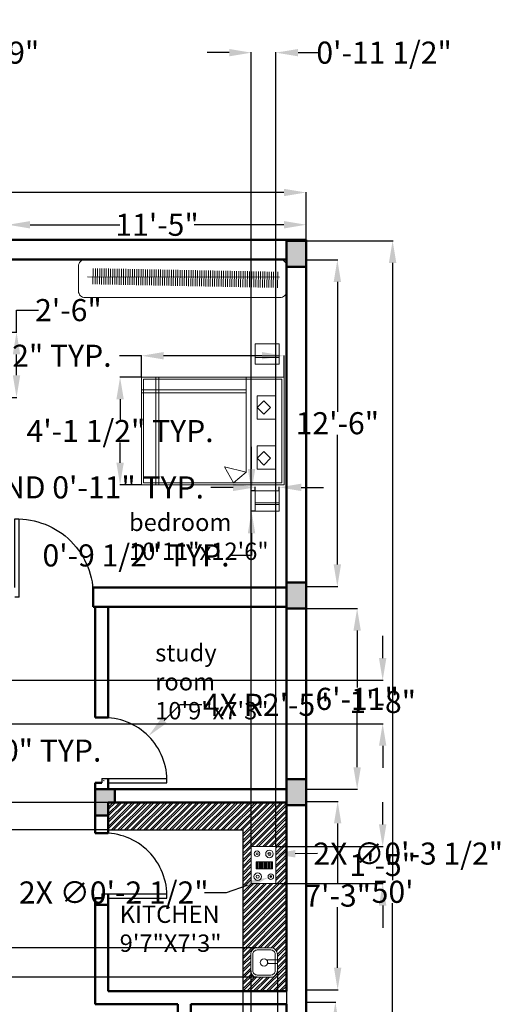
# Model space of a CAD drawing. Units: inches. Extents: x 22 to 1000, y 8 to 1043.
# Tile 3 of 3: x 779 to 1000, y 590 to 1043. Entities that reach past the tile are written whole.
import ezdxf

# ---------------------------------------------------------------- set-up
doc = ezdxf.new("R2010")
doc.units = ezdxf.units.IN
doc.header["$MEASUREMENT"] = 0
for name, color, linetype, lineweight in [('A-ANNO-DIMS', 2, 'Continuous', 18), ('A-AREA-IDEN', 7, 'Continuous', 25), ('A-COLS', 7, 'Continuous', 50), ('A-COLS-PATT', 1, 'Continuous', 13), ('A-CSWK', 30, 'Continuous', 25), ('A-DOOR', 4, 'Continuous', 25), ('A-EQPM', 9, 'Continuous', 18), ('A-EQPM-PATT', 9, 'Continuous', 13), ('A-FLOR-FIXT', 9, 'Continuous', 18), ('A-FURN', 8, 'Continuous', 18), ('A-FURN-PATT', 8, 'Continuous', 13), ('A-WALL', 7, 'Continuous', 50)]:
    doc.layers.add(name, color=color, linetype=linetype, lineweight=lineweight)
doc.layers.add('A-CSWK-PATT', color=143, linetype='Continuous', lineweight=13, true_color=0x7aafdf)
doc.styles.get("Standard").update_dxf_attribs({"font": 'arial.ttf'})
doc.dimstyles.get("Standard").update_dxf_attribs({"dimtxt": 10.18, "dimasz": 10.18, "dimexe": 0.18, "dimexo": 0.0625, "dimgap": 0.09, "dimtad": 0, "dimtih": 1, "dimtoh": 1, "dimdec": 0, "dimzin": 0, "dimdsep": 46, "dimlunit": 3, "dimtxsty": 'Standard', "dimcen": 0.09, "dimadec": 0, "dimazin": 0, "dimtfac": 1, "dimtdec": 0, "dimtofl": 0, "dimtmove": 0, "dimatfit": 3, "dimfxl": 1, "dimtolj": 1, "dimtzin": 0, "dimarcsym": 0})

# ---------------------------------------------------------------- blocks, each defined once
blk = doc.blocks.new('*D7')
at = {"layer": 'A-ANNO-DIMS', "color": 0, "lineweight": -2, "transparency": 16777216}
for p, q in [((773.8, 941.72), (773.8, 948.83)), ((783.98, 948.65), (825.3, 948.65)), ((900.81, 948.65), (859.49, 948.65)), ((910.99, 941.72), (910.99, 948.83))]:
    blk.add_line(p, q, dxfattribs=at)
at = {"layer": 'A-ANNO-DIMS', "color": 0, "transparency": 16777216}
for points in [[(783.98, 950.35), (783.98, 946.95), (773.8, 948.65)], [(900.81, 950.35), (900.81, 946.95), (910.99, 948.65)]]:
    blk.add_solid(points, dxfattribs=at)
at = {"layer": 'Defpoints', "color": 0, "transparency": 16777216}
for p in [(910.99, 948.65), (773.8, 941.66), (910.99, 941.66)]:
    blk.add_point(p, dxfattribs=at)
at = {"layer": 'A-ANNO-DIMS', "color": 0, "transparency": 16777216, "insert": (842.39, 948.65), "char_height": 10.18, "attachment_point": 5}
blk.add_mtext('\\A1;11\'-5"', dxfattribs=at)
blk = doc.blocks.new('*D14')
at = {"layer": 'A-ANNO-DIMS', "color": 0, "lineweight": -2, "transparency": 16777216}
for p, q in [((911.05, 590.68), (924.64, 590.68)), ((924.46, 580.5), (924.46, 471.45)), ((924.46, 351.84), (924.46, 460.88)), ((911.05, 341.66), (924.64, 341.66))]:
    blk.add_line(p, q, dxfattribs=at)
at = {"layer": 'A-ANNO-DIMS', "color": 0, "transparency": 16777216}
for points in [[(922.77, 580.5), (926.16, 580.5), (924.46, 590.68)], [(922.77, 351.84), (926.16, 351.84), (924.46, 341.66)]]:
    blk.add_solid(points, dxfattribs=at)
at = {"layer": 'Defpoints', "color": 0, "transparency": 16777216}
for p in [(910.99, 590.68), (924.46, 590.68), (910.99, 341.66)]:
    blk.add_point(p, dxfattribs=at)
at = {"layer": 'A-ANNO-DIMS', "color": 0, "transparency": 16777216, "insert": (924.46, 466.17), "char_height": 10.18, "attachment_point": 5}
blk.add_mtext('\\A1;20\'-9"', dxfattribs=at)
blk = doc.blocks.new('*D15')
at = {"layer": 'A-ANNO-DIMS', "color": 0, "lineweight": -2, "transparency": 16777216}
for p, q in [((911.05, 683.11), (925.7, 683.11)), ((925.52, 672.93), (925.52, 645.01)), ((925.52, 606.51), (925.52, 634.43)), ((911.05, 596.33), (925.7, 596.33))]:
    blk.add_line(p, q, dxfattribs=at)
at = {"layer": 'A-ANNO-DIMS', "color": 0, "transparency": 16777216}
for points in [[(923.82, 672.93), (927.22, 672.93), (925.52, 683.11)], [(923.82, 606.51), (927.22, 606.51), (925.52, 596.33)]]:
    blk.add_solid(points, dxfattribs=at)
at = {"layer": 'Defpoints', "color": 0, "transparency": 16777216}
for p in [(910.99, 683.11), (925.52, 683.11), (910.99, 596.33)]:
    blk.add_point(p, dxfattribs=at)
at = {"layer": 'A-ANNO-DIMS', "color": 0, "transparency": 16777216, "insert": (925.52, 639.72), "char_height": 10.18, "attachment_point": 5}
blk.add_mtext('\\A1;7\'-3"', dxfattribs=at)
blk = doc.blocks.new('*D16')
at = {"layer": 'A-ANNO-DIMS', "color": 0, "lineweight": -2, "transparency": 16777216}
for p, q in [((911.05, 771.96), (934.67, 771.96)), ((934.49, 761.78), (934.49, 735.6)), ((934.49, 698.84), (934.49, 725.02)), ((911.05, 688.66), (934.67, 688.66))]:
    blk.add_line(p, q, dxfattribs=at)
at = {"layer": 'A-ANNO-DIMS', "color": 0, "transparency": 16777216}
for points in [[(932.79, 761.78), (936.19, 761.78), (934.49, 771.96)], [(932.79, 698.84), (936.19, 698.84), (934.49, 688.66)]]:
    blk.add_solid(points, dxfattribs=at)
at = {"layer": 'Defpoints', "color": 0, "transparency": 16777216}
for p in [(910.99, 771.96), (934.49, 771.96), (910.99, 688.66)]:
    blk.add_point(p, dxfattribs=at)
at = {"layer": 'A-ANNO-DIMS', "color": 0, "transparency": 16777216, "insert": (934.49, 730.31), "char_height": 10.18, "attachment_point": 5}
blk.add_mtext('\\A1;6\'-11"', dxfattribs=at)
blk = doc.blocks.new('*D17')
at = {"layer": 'A-ANNO-DIMS', "color": 0, "lineweight": -2, "transparency": 16777216}
for p, q in [((911.05, 932.48), (925.56, 932.48)), ((925.38, 922.3), (925.38, 862.54)), ((925.38, 792.2), (925.38, 851.96)), ((911.05, 782.02), (925.56, 782.02))]:
    blk.add_line(p, q, dxfattribs=at)
at = {"layer": 'A-ANNO-DIMS', "color": 0, "transparency": 16777216}
for points in [[(923.68, 922.3), (927.08, 922.3), (925.38, 932.48)], [(923.68, 792.2), (927.08, 792.2), (925.38, 782.02)]]:
    blk.add_solid(points, dxfattribs=at)
at = {"layer": 'Defpoints', "color": 0, "transparency": 16777216}
for p in [(910.99, 932.48), (925.38, 932.48), (910.99, 782.02)]:
    blk.add_point(p, dxfattribs=at)
at = {"layer": 'A-ANNO-DIMS', "color": 0, "transparency": 16777216, "insert": (925.38, 857.25), "char_height": 10.18, "attachment_point": 5}
blk.add_mtext('\\A1;12\'-6"', dxfattribs=at)
blk = doc.blocks.new('*D20')
at = {"layer": 'A-ANNO-DIMS', "color": 0, "lineweight": -2, "transparency": 16777216}
for p, q in [((777.71, 899.16), (777.71, 909.34)), ((777.71, 909.34), (787.89, 909.34)), ((774.05, 899.16), (777.89, 899.16)), ((777.71, 879.34), (777.71, 888.98)), ((774.05, 869.16), (777.89, 869.16))]:
    blk.add_line(p, q, dxfattribs=at)
at = {"layer": 'A-ANNO-DIMS', "color": 0, "transparency": 16777216}
for points in [[(776.01, 888.98), (779.41, 888.98), (777.71, 899.16)], [(776.01, 879.34), (779.41, 879.34), (777.71, 869.16)]]:
    blk.add_solid(points, dxfattribs=at)
at = {"layer": 'Defpoints', "color": 0, "transparency": 16777216}
for p in [(773.99, 899.16), (777.71, 899.16), (773.99, 869.16)]:
    blk.add_point(p, dxfattribs=at)
at = {"layer": 'A-ANNO-DIMS', "color": 0, "transparency": 16777216, "insert": (801.6, 909.34), "char_height": 10.18, "attachment_point": 5}
blk.add_mtext('\\A1;2\'-6"', dxfattribs=at)
blk = doc.blocks.new('*D22')
at = {"layer": 'A-ANNO-DIMS', "color": 0, "lineweight": -2, "transparency": 16777216}
for p, q in [((550.99, 941.72), (550.99, 963.68)), ((561.17, 963.5), (722.27, 963.5)), ((900.81, 963.5), (739.72, 963.5)), ((910.99, 941.35), (910.99, 963.68))]:
    blk.add_line(p, q, dxfattribs=at)
at = {"layer": 'A-ANNO-DIMS', "color": 0, "transparency": 16777216}
for points in [[(561.17, 965.2), (561.17, 961.81), (550.99, 963.5)], [(900.81, 965.2), (900.81, 961.81), (910.99, 963.5)]]:
    blk.add_solid(points, dxfattribs=at)
at = {"layer": 'Defpoints', "color": 0, "transparency": 16777216}
for p in [(910.99, 963.5), (550.99, 941.66), (910.99, 941.29)]:
    blk.add_point(p, dxfattribs=at)
at = {"layer": 'A-ANNO-DIMS', "color": 0, "transparency": 16777216, "insert": (730.99, 963.5), "char_height": 10.18, "attachment_point": 5}
blk.add_mtext("\\A1;30'", dxfattribs=at)
blk = doc.blocks.new('*D23')
at = {"layer": 'A-ANNO-DIMS', "color": 0, "lineweight": -2, "transparency": 16777216}
for p, q in [((911.05, 941.29), (951, 941.29)), ((950.82, 931.11), (950.82, 646.76)), ((950.82, 351.84), (950.82, 636.18)), ((911.12, 341.66), (951, 341.66))]:
    blk.add_line(p, q, dxfattribs=at)
at = {"layer": 'A-ANNO-DIMS', "color": 0, "transparency": 16777216}
for points in [[(949.12, 931.11), (952.52, 931.11), (950.82, 941.29)], [(949.12, 351.84), (952.52, 351.84), (950.82, 341.66)]]:
    blk.add_solid(points, dxfattribs=at)
at = {"layer": 'Defpoints', "color": 0, "transparency": 16777216}
for p in [(910.99, 941.29), (911.05, 341.66), (950.82, 341.66)]:
    blk.add_point(p, dxfattribs=at)
at = {"layer": 'A-ANNO-DIMS', "color": 0, "transparency": 16777216, "insert": (950.82, 641.47), "char_height": 10.18, "attachment_point": 5}
blk.add_mtext("\\A1;50'", dxfattribs=at)
blk = doc.blocks.new('BED-DOUBLE')
for p, q in [((17.39, 43.76), (23.24, 48.65)), ((23.24, 48.65), (27.45, 41.36)), ((57.59, 49.65), (57.59, 0)), ((59, 49.65), (59, 0)), ((17.39, 0), (17.39, 43.76)), ((27.45, 41.36), (17.39, 43.76)), ((65.63, 7.18), (17.39, 7.18)), ((65.63, 5.85), (17.39, 5.85))]:
    blk.add_line(p, q)
for points in [[(0, 49.65), (65.63, 49.65), (65.63, 0), (0, 0)], [(1, 48.65), (64.63, 48.65), (64.63, 1), (1, 1)], [(3.82, 42.37), (12.46, 42.37), (12.46, 31.72), (3.82, 31.72)], [(9.34, 40.5), (6.22, 37.37), (9.34, 34.25), (12.46, 37.37)], [(3.82, 19.31), (12.46, 19.31), (12.46, 8.66), (3.82, 8.66)], [(9.34, 17.11), (6.22, 13.99), (9.34, 10.87), (12.46, 13.99)]]:
    blk.add_lwpolyline(points, close=True)
blk = doc.blocks.new('NIGHTSTAND')
for p, q in [((1.74, 9.32), (1.74, 0)), ((0, 6.3), (11.07, 6.3)), ((0, 5.43), (11.07, 5.43))]:
    blk.add_line(p, q)
blk.add_lwpolyline([(0, 9.32), (11.07, 9.32), (11.07, 0), (0, 0)], close=True)
blk = doc.blocks.new('DOOR-SWING-30IN')
for p, q in [((27.02, 30.02), (0.02, 30.02)), ((30.02, 28.02), (0.02, 28.02)), ((30.02, 28.02), (30.02, 30.02))]:
    blk.add_line(p, q)
blk.add_arc((29.02, 29.02), 29.02, 178.0251, 271.9749)
blk = doc.blocks.new('DOOR-SWING-36IN')
for p, q in [((34.01, 0), (34.01, 36)), ((36.01, 4.5), (36.01, 36)), ((34.01, 0), (36.01, 0))]:
    blk.add_line(p, q)
blk.add_arc((35.01, 1), 35.01, 88.3634, 181.6366)
blk = doc.blocks.new('COLUMN-9X12IN')
for p, q in [((0, 12), (9, 12)), ((0, 0), (0, 12)), ((9, 12), (9, 0)), ((9, 0), (0, 0))]:
    blk.add_line(p, q)
blk = doc.blocks.new('BURNER-LARGE')
for radius in [1.73, 0.692]:
    blk.add_circle((1.73, 1.73), radius)
blk = doc.blocks.new('BURNER-SMALL')
for radius in [1.27, 0.459]:
    blk.add_circle((1.27, 1.27), radius)
blk = doc.blocks.new('*D35')
at = {"layer": 'A-ANNO-DIMS', "color": 0, "lineweight": -2, "transparency": 16777216}
for p, q in [((877.36, 827.71), (867.18, 827.71)), ((887.54, 826.12), (887.54, 827.89)), ((898.61, 826.12), (898.61, 827.89)), ((908.79, 827.71), (918.97, 827.71))]:
    blk.add_line(p, q, dxfattribs=at)
at = {"layer": 'A-ANNO-DIMS', "color": 0, "transparency": 16777216}
for points in [[(877.36, 829.41), (877.36, 826.02), (887.54, 827.71)], [(908.79, 829.41), (908.79, 826.02), (898.61, 827.71)]]:
    blk.add_solid(points, dxfattribs=at)
at = {"layer": 'Defpoints', "color": 0, "transparency": 16777216}
for p in [(887.54, 827.71), (887.54, 826.05), (898.61, 826.05)]:
    blk.add_point(p, dxfattribs=at)
at = {"layer": 'A-ANNO-DIMS', "color": 0, "transparency": 16777216, "insert": (784.16, 827.71), "char_height": 10.18, "attachment_point": 5}
blk.add_mtext('\\A1;NIGHTSTAND 0\'-11" TYP.', dxfattribs=at)
blk = doc.blocks.new('*D36')
at = {"layer": 'A-ANNO-DIMS', "color": 0, "lineweight": -2, "transparency": 16777216}
for p, q in [((885.88, 836.23), (885.88, 846.41)), ((887.48, 826.05), (885.7, 826.05)), ((887.48, 816.74), (885.7, 816.74)), ((885.88, 806.56), (885.88, 796.38)), ((885.88, 796.38), (875.7, 796.38))]:
    blk.add_line(p, q, dxfattribs=at)
at = {"layer": 'A-ANNO-DIMS', "color": 0, "transparency": 16777216}
for points in [[(884.18, 836.23), (887.58, 836.23), (885.88, 826.05)], [(884.18, 806.56), (887.58, 806.56), (885.88, 816.74)]]:
    blk.add_solid(points, dxfattribs=at)
at = {"layer": 'Defpoints', "color": 0, "transparency": 16777216}
for p in [(887.54, 826.05), (885.88, 816.74), (887.54, 816.74)]:
    blk.add_point(p, dxfattribs=at)
at = {"layer": 'A-ANNO-DIMS', "color": 0, "transparency": 16777216, "insert": (832.72, 796.38), "char_height": 10.18, "attachment_point": 5}
blk.add_mtext('\\A1;0\'-9 1/2" TYP.', dxfattribs=at)
blk = doc.blocks.new('*D37')
at = {"layer": 'A-ANNO-DIMS', "color": 0, "lineweight": -2, "transparency": 16777216}
for p, q in [((618.65, 707.96), (618.65, 706.33)), ((628.76, 707.96), (628.76, 706.33)), ((608.47, 706.51), (598.29, 706.51)), ((638.94, 706.51), (649.12, 706.51))]:
    blk.add_line(p, q, dxfattribs=at)
at = {"layer": 'A-ANNO-DIMS', "color": 0, "transparency": 16777216}
for points in [[(608.47, 708.2), (608.47, 704.81), (618.65, 706.51)], [(638.94, 708.2), (638.94, 704.81), (628.76, 706.51)]]:
    blk.add_solid(points, dxfattribs=at)
at = {"layer": 'Defpoints', "color": 0, "transparency": 16777216}
for p in [(618.65, 708.02), (628.76, 708.02), (628.76, 706.51)]:
    blk.add_point(p, dxfattribs=at)
at = {"layer": 'A-ANNO-DIMS', "color": 0, "transparency": 16777216, "insert": (734.9, 706.51), "char_height": 10.18, "attachment_point": 5}
blk.add_mtext('\\A1;DINING CHAIR 0\'-10" TYP.', dxfattribs=at)
blk = doc.blocks.new('*D39')
at = {"layer": 'A-ANNO-DIMS', "color": 0, "lineweight": -2, "transparency": 16777216}
for p, q in [((835.23, 888.33), (825.05, 888.33)), ((835.23, 878.55), (835.23, 888.51)), ((890.68, 888.33), (845.41, 888.33)), ((900.86, 878.55), (900.86, 888.51))]:
    blk.add_line(p, q, dxfattribs=at)
at = {"layer": 'A-ANNO-DIMS', "color": 0, "transparency": 16777216}
for points in [[(845.41, 890.03), (845.41, 886.64), (835.23, 888.33)], [(890.68, 890.03), (890.68, 886.64), (900.86, 888.33)]]:
    blk.add_solid(points, dxfattribs=at)
at = {"layer": 'Defpoints', "color": 0, "transparency": 16777216}
for p in [(835.23, 888.33), (835.23, 878.49), (900.86, 878.49)]:
    blk.add_point(p, dxfattribs=at)
at = {"layer": 'A-ANNO-DIMS', "color": 0, "transparency": 16777216, "insert": (734.51, 888.33), "char_height": 10.18, "attachment_point": 5}
blk.add_mtext('\\A1;DOUBLE BED 5\'-5 1/2" TYP.', dxfattribs=at)
blk = doc.blocks.new('*D40')
at = {"layer": 'A-ANNO-DIMS', "color": 0, "lineweight": -2, "transparency": 16777216}
for p, q in [((835.16, 878.49), (825.2, 878.49)), ((825.38, 868.31), (825.38, 859.02)), ((825.38, 839.02), (825.38, 848.31)), ((835.16, 828.84), (825.2, 828.84))]:
    blk.add_line(p, q, dxfattribs=at)
at = {"layer": 'A-ANNO-DIMS', "color": 0, "transparency": 16777216}
for points in [[(823.68, 868.31), (827.08, 868.31), (825.38, 878.49)], [(823.68, 839.02), (827.08, 839.02), (825.38, 828.84)]]:
    blk.add_solid(points, dxfattribs=at)
at = {"layer": 'Defpoints', "color": 0, "transparency": 16777216}
for p in [(835.23, 878.49), (825.38, 828.84), (835.23, 828.84)]:
    blk.add_point(p, dxfattribs=at)
at = {"layer": 'A-ANNO-DIMS', "color": 0, "transparency": 16777216, "insert": (825.38, 853.66), "char_height": 10.18, "attachment_point": 5}
blk.add_mtext('\\A1;4\'-1 1/2" TYP.', dxfattribs=at)
blk = doc.blocks.new('*D46')
at = {"layer": 'A-ANNO-DIMS', "color": 0, "lineweight": -2, "transparency": 16777216}
for p, q in [((875.6, 1027.91), (865.42, 1027.91)), ((885.78, 662.39), (885.78, 1028.09)), ((897.1, 662.39), (897.1, 1028.09)), ((907.28, 1027.91), (917.46, 1027.91))]:
    blk.add_line(p, q, dxfattribs=at)
at = {"layer": 'A-ANNO-DIMS', "color": 0, "transparency": 16777216}
for points in [[(875.6, 1029.6), (875.6, 1026.21), (885.78, 1027.91)], [(907.28, 1029.6), (907.28, 1026.21), (897.1, 1027.91)]]:
    blk.add_solid(points, dxfattribs=at)
at = {"layer": 'Defpoints', "color": 0, "transparency": 16777216}
for p in [(897.1, 1027.91), (885.78, 662.33), (897.1, 662.33)]:
    blk.add_point(p, dxfattribs=at)
at = {"layer": 'A-ANNO-DIMS', "color": 0, "transparency": 16777216, "insert": (946.89, 1027.91), "char_height": 10.18, "attachment_point": 5}
blk.add_mtext('\\A1;0\'-11 1/2"', dxfattribs=at)
blk = doc.blocks.new('*D47')
at = {"layer": 'A-ANNO-DIMS', "color": 0, "lineweight": -2, "transparency": 16777216}
for p, q in [((946.24, 672.51), (946.24, 682.69)), ((897.16, 662.33), (946.42, 662.33)), ((897.16, 645.29), (946.42, 645.29)), ((946.24, 635.11), (946.24, 624.93))]:
    blk.add_line(p, q, dxfattribs=at)
at = {"layer": 'A-ANNO-DIMS', "color": 0, "transparency": 16777216}
for points in [[(944.54, 672.51), (947.94, 672.51), (946.24, 662.33)], [(944.54, 635.11), (947.94, 635.11), (946.24, 645.29)]]:
    blk.add_solid(points, dxfattribs=at)
at = {"layer": 'Defpoints', "color": 0, "transparency": 16777216}
for p in [(897.1, 662.33), (946.24, 662.33), (897.1, 645.29)]:
    blk.add_point(p, dxfattribs=at)
at = {"layer": 'A-ANNO-DIMS', "color": 0, "transparency": 16777216, "insert": (946.24, 653.81), "char_height": 10.18, "attachment_point": 5}
blk.add_mtext('\\A1;1\'-5"', dxfattribs=at)
blk = doc.blocks.new('*D48')
at = {"layer": 'A-ANNO-DIMS', "color": 0, "lineweight": -2, "transparency": 16777216}
for p, q in [((881.83, 595.59), (881.83, 289.9)), ((901.99, 595.59), (901.99, 289.9)), ((871.65, 290.08), (861.47, 290.08)), ((912.17, 290.08), (922.35, 290.08))]:
    blk.add_line(p, q, dxfattribs=at)
at = {"layer": 'A-ANNO-DIMS', "color": 0, "transparency": 16777216}
for points in [[(871.65, 291.77), (871.65, 288.38), (881.83, 290.08)], [(912.17, 291.77), (912.17, 288.38), (901.99, 290.08)]]:
    blk.add_solid(points, dxfattribs=at)
at = {"layer": 'Defpoints', "color": 0, "transparency": 16777216}
for p in [(881.83, 595.66), (901.99, 595.66), (901.99, 290.08)]:
    blk.add_point(p, dxfattribs=at)
at = {"layer": 'A-ANNO-DIMS', "color": 0, "transparency": 16777216, "insert": (935.49, 290.08), "char_height": 10.18, "attachment_point": 5}
blk.add_mtext('\\A1;1\'-8"', dxfattribs=at)
blk = doc.blocks.new('*D49')
at = {"layer": 'A-ANNO-DIMS', "color": 0, "lineweight": -2, "transparency": 16777216}
for p, q in [((515.74, 692.84), (515.74, 703.02)), ((819.86, 682.66), (515.56, 682.66)), ((819.86, 669.94), (515.56, 669.94)), ((515.74, 659.76), (515.74, 649.58))]:
    blk.add_line(p, q, dxfattribs=at)
at = {"layer": 'A-ANNO-DIMS', "color": 0, "transparency": 16777216}
for points in [[(514.04, 692.84), (517.44, 692.84), (515.74, 682.66)], [(514.04, 659.76), (517.44, 659.76), (515.74, 669.94)]]:
    blk.add_solid(points, dxfattribs=at)
at = {"layer": 'Defpoints', "color": 0, "transparency": 16777216}
for p in [(515.74, 682.66), (819.92, 682.66), (819.92, 669.94)]:
    blk.add_point(p, dxfattribs=at)
at = {"layer": 'A-ANNO-DIMS', "color": 0, "transparency": 16777216, "insert": (515.74, 676.3), "char_height": 10.18, "attachment_point": 5}
blk.add_mtext('\\A1;1\'-0 1/2"', dxfattribs=at)
blk = doc.blocks.new('*D50')
at = {"layer": 'A-ANNO-DIMS', "color": 0, "lineweight": -2, "transparency": 16777216}
for p, q in [((885.49, 605.07), (885.49, 289.9)), ((897.78, 605.07), (897.78, 289.9)), ((875.31, 290.08), (865.13, 290.08)), ((907.96, 290.08), (918.14, 290.08))]:
    blk.add_line(p, q, dxfattribs=at)
at = {"layer": 'A-ANNO-DIMS', "color": 0, "transparency": 16777216}
for points in [[(875.31, 291.77), (875.31, 288.38), (885.49, 290.08)], [(907.96, 291.77), (907.96, 288.38), (897.78, 290.08)]]:
    blk.add_solid(points, dxfattribs=at)
at = {"layer": 'Defpoints', "color": 0, "transparency": 16777216}
for p in [(885.49, 605.13), (897.78, 605.13), (897.78, 290.08)]:
    blk.add_point(p, dxfattribs=at)
at = {"layer": 'A-ANNO-DIMS', "color": 0, "transparency": 16777216, "insert": (943.14, 290.08), "char_height": 10.18, "attachment_point": 5}
blk.add_mtext('\\A1;1\'-0 1/2"', dxfattribs=at)
blk = doc.blocks.new('*D51')
at = {"layer": 'A-ANNO-DIMS', "color": 0, "lineweight": -2, "transparency": 16777216}
for p, q in [((515.74, 625.87), (515.74, 636.05)), ((888.43, 615.69), (515.56, 615.69)), ((888.43, 602.13), (515.56, 602.13)), ((515.74, 591.95), (515.74, 581.77))]:
    blk.add_line(p, q, dxfattribs=at)
at = {"layer": 'A-ANNO-DIMS', "color": 0, "transparency": 16777216}
for points in [[(514.04, 625.87), (517.44, 625.87), (515.74, 615.69)], [(514.04, 591.95), (517.44, 591.95), (515.74, 602.13)]]:
    blk.add_solid(points, dxfattribs=at)
at = {"layer": 'Defpoints', "color": 0, "transparency": 16777216}
for p in [(515.74, 615.69), (888.49, 615.69), (888.49, 602.13)]:
    blk.add_point(p, dxfattribs=at)
at = {"layer": 'A-ANNO-DIMS', "color": 0, "transparency": 16777216, "insert": (515.74, 608.91), "char_height": 10.18, "attachment_point": 5}
blk.add_mtext('\\A1;1\'-1 1/2"', dxfattribs=at)
blk = doc.blocks.new('*D52')
at = {"layer": 'A-ANNO-DIMS', "color": 0, "lineweight": -2, "transparency": 16777216}
for p, q in [((728.5, 932.72), (728.5, 1028.09)), ((738.68, 1027.91), (739.32, 1027.91)), ((749.5, 932.72), (749.5, 1028.09)), ((749.5, 1027.91), (759.68, 1027.91))]:
    blk.add_line(p, q, dxfattribs=at)
at = {"layer": 'A-ANNO-DIMS', "color": 0, "transparency": 16777216}
for points in [[(738.68, 1029.6), (738.68, 1026.21), (728.5, 1027.91)], [(739.32, 1029.6), (739.32, 1026.21), (749.5, 1027.91)]]:
    blk.add_solid(points, dxfattribs=at)
at = {"layer": 'Defpoints', "color": 0, "transparency": 16777216}
for p in [(749.5, 1027.91), (728.5, 932.66), (749.5, 932.66)]:
    blk.add_point(p, dxfattribs=at)
at = {"layer": 'A-ANNO-DIMS', "color": 0, "transparency": 16777216, "insert": (772.82, 1027.91), "char_height": 10.18, "attachment_point": 5}
blk.add_mtext('\\A1;1\'-9"', dxfattribs=at)
blk = doc.blocks.new('*D55')
at = {"layer": 'A-ANNO-DIMS', "color": 0, "lineweight": -2, "transparency": 16777216}
for p, q in [((946.24, 749.09), (946.24, 759.27)), ((631.37, 738.91), (946.42, 738.91)), ((631.37, 718.87), (946.42, 718.87)), ((946.24, 708.69), (946.24, 698.51))]:
    blk.add_line(p, q, dxfattribs=at)
at = {"layer": 'A-ANNO-DIMS', "color": 0, "transparency": 16777216}
for points in [[(944.54, 749.09), (947.94, 749.09), (946.24, 738.91)], [(944.54, 708.69), (947.94, 708.69), (946.24, 718.87)]]:
    blk.add_solid(points, dxfattribs=at)
at = {"layer": 'Defpoints', "color": 0, "transparency": 16777216}
for p in [(631.31, 738.91), (946.24, 738.91), (631.31, 718.87)]:
    blk.add_point(p, dxfattribs=at)
at = {"layer": 'A-ANNO-DIMS', "color": 0, "transparency": 16777216, "insert": (946.24, 728.89), "char_height": 10.18, "attachment_point": 5}
blk.add_mtext('\\A1;1\'-8"', dxfattribs=at)
blk = doc.blocks.new('*D59')
at = {"layer": 'A-ANNO-DIMS', "color": 0, "lineweight": -2, "transparency": 16777216}
for p, q in [((852.84, 727.57), (845.64, 720.37)), ((863.02, 727.57), (852.84, 727.57)), ((817.83, 692.66), (818.01, 692.66)), ((817.92, 692.57), (817.92, 692.75))]:
    blk.add_line(p, q, dxfattribs=at)
at = {"layer": 'A-ANNO-DIMS', "color": 0, "transparency": 16777216}
blk.add_solid([(844.44, 721.57), (846.84, 719.17), (838.44, 713.18)], dxfattribs=at)
at = {"layer": 'Defpoints', "color": 0, "transparency": 16777216}
for p in [(838.44, 713.18), (817.92, 692.66)]:
    blk.add_point(p, dxfattribs=at)
at = {"layer": 'A-ANNO-DIMS', "color": 0, "transparency": 16777216, "insert": (892.65, 727.57), "char_height": 10.18, "attachment_point": 5}
blk.add_mtext('\\A1;4X R2\'-5"', dxfattribs=at)
blk = doc.blocks.new('*D63')
at = {"layer": 'A-ANNO-DIMS', "color": 0, "lineweight": -2, "transparency": 16777216}
for p, q in [((894.04, 658.89), (894.22, 658.89)), ((894.13, 658.8), (894.13, 658.98)), ((916.22, 659.06), (906.04, 658.98))]:
    blk.add_line(p, q, dxfattribs=at)
at = {"layer": 'A-ANNO-DIMS', "color": 0, "transparency": 16777216}
blk.add_solid([(906.02, 660.68), (906.05, 657.28), (895.86, 658.9)], dxfattribs=at)
at = {"layer": 'Defpoints', "color": 0, "transparency": 16777216}
for p in [(892.4, 658.87), (895.86, 658.9)]:
    blk.add_point(p, dxfattribs=at)
at = {"layer": 'A-ANNO-DIMS', "color": 0, "transparency": 16777216, "insert": (957.99, 659.06), "char_height": 10.18, "attachment_point": 5}
blk.add_mtext('\\A1;2X ∅0\'-3 1/2"', dxfattribs=at)
blk = doc.blocks.new('*D64')
at = {"layer": 'A-ANNO-DIMS', "color": 0, "lineweight": -2, "transparency": 16777216}
for p, q in [((894.68, 648.46), (894.86, 648.46)), ((894.77, 648.37), (894.77, 648.55)), ((874.41, 641.15), (883.99, 644.59)), ((864.23, 641.15), (874.41, 641.15))]:
    blk.add_line(p, q, dxfattribs=at)
at = {"layer": 'A-ANNO-DIMS', "color": 0, "transparency": 16777216}
blk.add_solid([(883.42, 646.19), (884.57, 642.99), (893.57, 648.03)], dxfattribs=at)
at = {"layer": 'Defpoints', "color": 0, "transparency": 16777216}
for p in [(895.96, 648.89), (893.57, 648.03)]:
    blk.add_point(p, dxfattribs=at)
at = {"layer": 'A-ANNO-DIMS', "color": 0, "transparency": 16777216, "insert": (822.46, 641.15), "char_height": 10.18, "attachment_point": 5}
blk.add_mtext('\\A1;2X ∅0\'-2 1/2"', dxfattribs=at)

msp = doc.modelspace()

# ---------------------------------------------------------------- hatches: boundary and pattern name
at = {"layer": 'A-COLS-PATT'}
h = msp.add_hatch(color=256, dxfattribs=at)
h.dxf.hatch_style = 1
h.paths.add_polyline_path([(559.99, 941.66), (550.99, 941.66), (550.99, 929.67), (559.99, 929.67)])
h.paths.add_polyline_path([(910.99, 941.29), (901.99, 941.29), (901.99, 929.29), (910.99, 929.29)])
h.paths.add_polyline_path([(910.99, 783.96), (901.99, 783.96), (901.99, 771.96), (910.99, 771.96)])
h.paths.add_polyline_path([(910.99, 693.33), (901.99, 693.33), (901.99, 681.33), (910.99, 681.33)])
h.paths.add_polyline_path([(910.99, 494.22), (901.99, 494.22), (901.99, 482.22), (910.99, 482.22)])
h.paths.add_polyline_path([(721.99, 362.66), (712.99, 362.66), (712.99, 350.66), (721.99, 350.66)])
h.paths.add_polyline_path([(721.99, 489.46), (712.99, 489.46), (712.99, 477.46), (721.99, 477.46)])
h.paths.add_polyline_path([(559.99, 353.66), (550.99, 353.66), (550.99, 341.66), (559.99, 341.66)])
h.paths.add_polyline_path([(559.99, 467.38), (550.99, 467.38), (550.99, 455.38), (559.99, 455.38)])
h.paths.add_polyline_path([(559.99, 784.66), (550.99, 784.66), (550.99, 772.66), (559.99, 772.66)])
h.paths.add_polyline_path([(715.99, 781.66), (712.99, 781.66), (712.99, 784.66), (706.99, 784.66), (706.99, 772.66), (715.99, 772.66)])
h.paths.add_polyline_path([(822.98, 688.66), (813.98, 688.66), (813.98, 676.66), (819.92, 676.66), (819.92, 682.66), (822.98, 682.66)])
at = {"layer": 'A-CSWK-PATT'}
h = msp.add_hatch(dxfattribs=at)
h.set_pattern_fill('ANSI32', color=256, scale=5.6)
h.paths.add_polyline_path([(901.99, 682.66), (819.92, 682.66), (819.92, 669.94), (881.83, 669.94), (881.83, 595.66), (901.99, 595.66)])
h.paths.add_polyline_path([(885.78, 662.33), (897.1, 662.33), (897.1, 645.29), (885.78, 645.29)], flags=16)
h.paths.add_polyline_path([(889.69, 659, -1), (887.15, 659, -1)], flags=0)
h.paths.add_polyline_path([(888.88, 659, -1), (887.97, 659, -1)], flags=0)
h.paths.add_polyline_path([(895.86, 658.89, -1), (892.4, 658.89, -1)], flags=0)
h.paths.add_polyline_path([(894.82, 658.89, -1), (893.44, 658.89, -1)], flags=0)
h.paths.add_polyline_path([(888.07, 655.33), (895.5, 655.33), (895.5, 652.11), (888.07, 652.11)], flags=0)
h.paths.add_polyline_path([(890.46, 648.44, -1), (887, 648.44, -1)], flags=0)
h.paths.add_polyline_path([(889.42, 648.44, -1), (888.04, 648.44, -1)], flags=0)
h.paths.add_polyline_path([(896.04, 648.46, -1), (893.5, 648.46, -1)], flags=0)
h.paths.add_polyline_path([(895.23, 648.46, -1), (894.31, 648.46, -1)], flags=0)
h.paths.add_polyline_path([(888.49, 615.69), (894.78, 615.69, -0.414214), (897.78, 612.69), (897.78, 605.13, -0.414214), (894.78, 602.13), (888.49, 602.13, -0.414214), (885.49, 605.13), (885.49, 612.69, -0.414214)], flags=16)
h.paths.add_polyline_path([(888.49, 614.69), (894.78, 614.69, -0.414214), (896.78, 612.69), (896.78, 610.07), (897.78, 610.07), (897.78, 608.39), (896.78, 608.39), (896.78, 605.13, -0.414214), (894.78, 603.13), (888.49, 603.13, -0.414214), (886.49, 605.13), (886.49, 612.69, -0.414214)], flags=0)
h.paths.add_polyline_path([(893.34, 608.91, -1), (889.92, 608.91, -1)], flags=0)
at = {"layer": 'A-EQPM-PATT'}
h = msp.add_hatch(dxfattribs=at)
h.set_pattern_fill('ANSI31', color=256, scale=4, angle=45, style=0)
h.paths.add_polyline_path([(888.07, 655.33), (895.5, 655.33), (895.5, 652.11), (888.07, 652.11)])
at = {"layer": 'A-FURN-PATT'}
h = msp.add_hatch(dxfattribs=at)
h.set_pattern_fill('ANSI31', color=256, scale=8, angle=43.8969, style=0)
h.paths.add_polyline_path([(812.83, 921.29), (898.81, 919.63), (898.95, 926.92), (812.97, 928.58)])

# ---------------------------------------------------------------- linework, layer by layer
at = {"layer": 'A-COLS'}
for p, q in [((813.98, 688.66), (822.98, 688.66)), ((813.98, 676.66), (813.98, 688.66)), ((822.98, 688.66), (822.98, 682.66)), ((819.92, 676.66), (813.98, 676.66))]:
    msp.add_line(p, q, dxfattribs=at)
at = {"layer": 'A-CSWK'}
for p, q in [((819.92, 669.94), (881.83, 669.94)), ((881.83, 669.94), (881.83, 595.66))]:
    msp.add_line(p, q, dxfattribs=at)
at = {"layer": 'A-EQPM'}
for points in [[(885.78, 662.33), (885.78, 662.33), (897.1, 662.33), (897.1, 662.33), (897.1, 645.29), (897.1, 645.29), (885.78, 645.29), (885.78, 645.29)], [(888.07, 655.33), (888.07, 655.33), (895.5, 655.33), (895.5, 655.33), (895.5, 652.11), (895.5, 652.11), (888.07, 652.11), (888.07, 652.11)]]:
    msp.add_lwpolyline(points, close=True, dxfattribs=at)
at = {"layer": 'A-FLOR-FIXT'}
for points in [[(885.49, 612.69, -0.414214), (888.49, 615.69), (894.78, 615.69, -0.414214), (897.78, 612.69), (897.78, 605.13, -0.414214), (894.78, 602.13), (888.49, 602.13, -0.414214), (885.49, 605.13)], [(886.49, 612.69, -0.414214), (888.49, 614.69), (894.78, 614.69, -0.414214), (896.78, 612.69), (896.78, 605.13, -0.414214), (894.78, 603.13), (888.49, 603.13, -0.414214), (886.49, 605.13)]]:
    msp.add_lwpolyline(points, format="xyb", close=True, dxfattribs=at)
msp.add_lwpolyline([(897.78, 610.07), (897.78, 610.07), (893.26, 610.07), (893.26, 610.07), (893.26, 608.39), (893.26, 608.39), (897.78, 608.39), (897.78, 608.39)], close=True, dxfattribs=at)
msp.add_circle((891.63, 608.91), 1.71, dxfattribs=at)
at = {"layer": 'A-FURN'}
msp.add_line((810.38, 924.64), (898.79, 924.5), dxfattribs=at)
msp.add_lwpolyline([(806.24, 929.66, -0.414214), (809.24, 932.66), (898.99, 932.66, -0.414214), (901.99, 929.66), (901.99, 918.09, -0.414214), (898.99, 915.09), (809.24, 915.09, -0.414214), (806.24, 918.09)], format="xyb", close=True, dxfattribs=at)
at = {"layer": 'A-WALL'}
for p, q in [((550.99, 941.66), (910.99, 941.66)), ((910.99, 941.66), (910.99, 341.66)), ((773.99, 932.66), (901.99, 932.66)), ((901.99, 932.66), (901.99, 781.66)), ((812.83, 781.66), (901.99, 781.66)), ((812.99, 781.66), (812.99, 772.66)), ((812.99, 772.66), (901.99, 772.66)), ((813.92, 772.66), (813.92, 721.66)), ((819.92, 772.66), (819.92, 721.61)), ((901.99, 772.66), (901.99, 688.66)), ((819.92, 721.66), (813.92, 721.66)), ((816.92, 691.66), (813.92, 691.66)), ((813.92, 691.66), (813.92, 668.53)), ((819.92, 693.66), (819.92, 688.66)), ((819.92, 688.66), (813.92, 688.66)), ((819.92, 688.66), (901.99, 688.66)), ((819.92, 682.66), (901.99, 682.66)), ((819.92, 682.66), (819.92, 668.48)), ((901.99, 682.66), (901.99, 595.66)), ((819.92, 668.53), (813.92, 668.53)), ((819.92, 640.53), (819.92, 595.66)), ((816.92, 638.53), (813.92, 638.53)), ((813.92, 638.53), (813.92, 589.66)), ((819.92, 635.53), (813.92, 635.53)), ((819.92, 595.66), (901.99, 595.66)), ((813.92, 589.66), (851.96, 589.66)), ((851.96, 589.66), (851.96, 464.66)), ((857.96, 589.66), (857.96, 458.66)), ((857.96, 589.66), (901.99, 589.66)), ((901.99, 589.66), (901.99, 350.66))]:
    msp.add_line(p, q, dxfattribs=at)

# ---------------------------------------------------------------- block references
at = {"layer": 'A-COLS'}
for p in [(901.99, 929.29), (901.99, 771.96), (901.99, 681.33)]:
    msp.add_blockref('COLUMN-9X12IN', p, dxfattribs=at)
at = {"layer": 'A-DOOR', "extrusion": (0, 0, -1), "zscale": -1}
msp.add_blockref('DOOR-SWING-36IN', (-813, 777.16), dxfattribs=at)
at = {"layer": 'A-DOOR', "rotation": 180}
for p in [(846.94, 721.67), (846.94, 668.54)]:
    msp.add_blockref('DOOR-SWING-30IN', p, dxfattribs=at)
at = {"layer": 'A-EQPM'}
for name, p in [('BURNER-SMALL', (887.15, 657.73)), ('BURNER-LARGE', (892.4, 657.16)), ('BURNER-LARGE', (887, 646.71)), ('BURNER-SMALL', (893.5, 647.19))]:
    msp.add_blockref(name, p, dxfattribs=at)
at = {"layer": 'A-FURN', "rotation": 180}
for name, p in [('NIGHTSTAND', (898.61, 893.79)), ('BED-DOUBLE', (900.86, 878.49)), ('NIGHTSTAND', (898.61, 826.05))]:
    msp.add_blockref(name, p, dxfattribs=at)

# ---------------------------------------------------------------- texts
at = {"layer": 'A-AREA-IDEN', "char_height": 8, "attachment_point": 1}
for s, width, insert in [('bedroom\\P10\'11"x12\'6"', 46.5585, (829.49, 815.62)), ('study room\\P10\'9"x7\'3"', 55.1173, (841.54, 755.54)), ('KITCHEN\\P9\'7"X7\'3"', 46.5585, (825.18, 635.15))]:
    msp.add_mtext_dynamic_manual_height_columns(s, width=width, gutter_width=1, heights=[0], dxfattribs=dict(at, insert=insert))

# ---------------------------------------------------------------- dimensions: what is measured, and where the dimension line sits
at = {"layer": 'A-ANNO-DIMS'}
for base, p1, p2, override, picture, middle in [((897.1, 1027.91), (885.78, 662.33), (897.1, 662.33), {"dimdec": 1, "dimlfac": 1, "dimrnd": 0, "dimzin": 1, "dimdsep": 46, "dimlunit": 4, "dimfrac": 2}, '*D46', (946.89, 1027.91)), ((749.5, 1027.91), (728.5, 932.66), (749.5, 932.66), {"dimdec": 1, "dimlfac": 1, "dimrnd": 0, "dimzin": 1, "dimdsep": 46, "dimlunit": 4, "dimfrac": 2}, '*D52', (772.82, 1027.91)), ((910.99, 963.5), (550.99, 941.66), (910.99, 941.29), {"dimclrd": 0, "dimclre": 0, "dimclrt": 0}, '*D22', (730.99, 963.5)), ((910.99, 948.65), (773.8, 941.66), (910.99, 941.66), {"dimclrd": 0, "dimclre": 0, "dimclrt": 0}, '*D7', (842.39, 948.65)), ((897.78, 290.08), (885.49, 605.13), (897.78, 605.13), {"dimdec": 1, "dimlfac": 1, "dimrnd": 0, "dimzin": 1, "dimdsep": 46, "dimlunit": 4, "dimfrac": 2}, '*D50', (943.14, 290.08)), ((901.99, 290.08), (881.83, 595.66), (901.99, 595.66), {"dimdec": 1, "dimlfac": 1, "dimrnd": 0, "dimzin": 1, "dimdsep": 46, "dimlunit": 4, "dimfrac": 2}, '*D48', (935.49, 290.08))]:
    dim = msp.add_linear_dim(base=base, p1=p1, p2=p2, dimstyle='Standard', override=override, dxfattribs=at)
    dim.commit()
    dim.dimension.update_dxf_attribs({"geometry": picture, "text_midpoint": middle})
for base, p1, p2, override, picture, middle in [((950.82, 341.66), (910.99, 941.29), (911.05, 341.66), {"dimclrd": 0, "dimclre": 0, "dimclrt": 0}, '*D23', (950.82, 641.47)), ((925.38, 932.48), (910.99, 782.02), (910.99, 932.48), {"dimclrd": 0, "dimclre": 0, "dimclrt": 0}, '*D17', (925.38, 857.25)), ((777.71, 899.16), (773.99, 869.16), (773.99, 899.16), {"dimclrd": 0, "dimclre": 0, "dimclrt": 0}, '*D20', (801.6, 909.34)), ((934.49, 771.96), (910.99, 688.66), (910.99, 771.96), {"dimclrd": 0, "dimclre": 0, "dimclrt": 0}, '*D16', (934.49, 730.31)), ((946.24, 738.91), (631.31, 718.87), (631.31, 738.91), {"dimdec": 1, "dimlfac": 1, "dimrnd": 0, "dimzin": 1, "dimdsep": 46, "dimlunit": 4, "dimfrac": 2}, '*D55', (946.24, 728.89)), ((515.74, 682.66), (819.92, 669.94), (819.92, 682.66), {"dimdec": 1, "dimlfac": 1, "dimrnd": 0, "dimzin": 1, "dimdsep": 46, "dimlunit": 4, "dimfrac": 2}, '*D49', (515.74, 676.3)), ((946.24, 662.33), (897.1, 645.29), (897.1, 662.33), {"dimdec": 1, "dimlfac": 1, "dimrnd": 0, "dimzin": 1, "dimdsep": 46, "dimlunit": 4, "dimfrac": 2}, '*D47', (946.24, 653.81)), ((925.52, 683.11), (910.99, 596.33), (910.99, 683.11), {"dimclrd": 0, "dimclre": 0, "dimclrt": 0}, '*D15', (925.52, 639.72)), ((515.74, 615.69), (888.49, 602.13), (888.49, 615.69), {"dimdec": 1, "dimlfac": 1, "dimrnd": 0, "dimzin": 1, "dimdsep": 46, "dimlunit": 4, "dimfrac": 2}, '*D51', (515.74, 608.91)), ((924.46, 590.68), (910.99, 341.66), (910.99, 590.68), {"dimclrd": 0, "dimclre": 0, "dimclrt": 0}, '*D14', (924.46, 466.17))]:
    dim = msp.add_linear_dim(base=base, p1=p1, p2=p2, angle=90, dimstyle='Standard', override=override, dxfattribs=at)
    dim.commit()
    dim.dimension.update_dxf_attribs({"geometry": picture, "text_midpoint": middle})
for base, p1, p2, angle, text, picture, middle in [((835.23, 888.33), (900.86, 878.49), (835.23, 878.49), 180, 'DOUBLE BED <> TYP.', '*D39', (734.51, 888.33)), ((825.3811, 828.8379), (835.2256, 878.4878), (835.2256, 828.8379), 270, '<> TYP.', '*D40', (825.3811, 853.6628)), ((887.54, 827.71), (898.61, 826.05), (887.54, 826.05), 180, 'NIGHTSTAND <> TYP.', '*D35', (784.16, 827.71)), ((885.88, 816.74), (887.54, 826.05), (887.54, 816.74), 270, '<> TYP.', '*D36', (832.72, 796.38))]:
    dim = msp.add_linear_dim(base=base, p1=p1, p2=p2, angle=angle, text=text, dimstyle='Standard', override={"dimdec": 1, "dimlfac": 1, "dimrnd": 0, "dimzin": 1, "dimdsep": 46, "dimlunit": 4, "dimfrac": 2}, dxfattribs=at)
    dim.commit()
    dim.dimension.update_dxf_attribs({"geometry": picture, "text_midpoint": middle})
dim = msp.add_radius_dim(center=(817.92, 692.66), mpoint=(838.44, 713.18), text='4X <>', dimstyle='Standard', override={"dimdec": 1, "dimlfac": 1, "dimrnd": 0, "dimzin": 1, "dimdsep": 46, "dimlunit": 4, "dimfrac": 2}, dxfattribs=at)
dim.commit()
dim.dimension.update_dxf_attribs({"geometry": '*D59', "text_midpoint": (892.65, 727.57)})
dim = msp.add_linear_dim(base=(628.76, 706.51), p1=(618.65, 708.02), p2=(628.76, 708.02), text='DINING CHAIR <> TYP.', dimstyle='Standard', override={"dimdec": 1, "dimlfac": 1, "dimrnd": 0, "dimzin": 1, "dimdsep": 46, "dimlunit": 4, "dimfrac": 2}, dxfattribs=at)
dim.commit()
dim.dimension.update_dxf_attribs({"geometry": '*D37', "text_midpoint": (734.9, 706.51)})
for p1, p2, picture, middle in [((892.4, 658.87), (895.86, 658.9), '*D63', (916.22, 659.06)), ((895.96, 648.89), (893.57, 648.03), '*D64', (822.46, 641.15))]:
    dim = msp.add_diameter_dim_2p(p1=p1, p2=p2, text='2X <>', dimstyle='Standard', override={"dimdec": 1, "dimlfac": 1, "dimrnd": 0, "dimzin": 1, "dimdsep": 46, "dimlunit": 4, "dimfrac": 2}, dxfattribs=at)
    dim.commit()
    dim.dimension.update_dxf_attribs({"geometry": picture, "text_midpoint": middle, "dimtype": 163})

doc.saveas('drawing.dxf')
